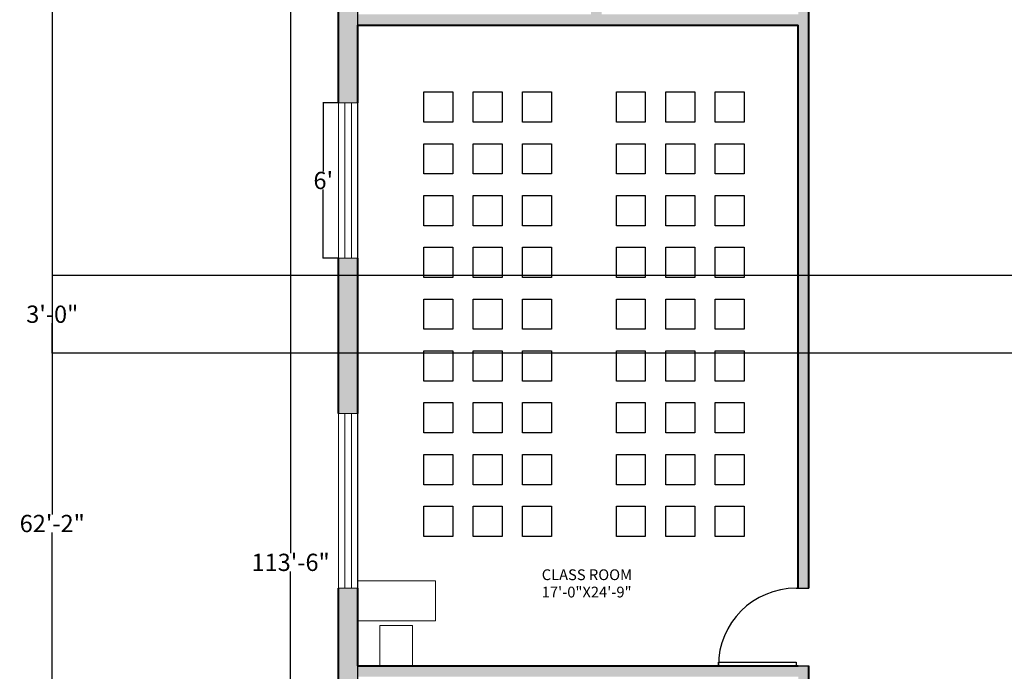
# Model space of a CAD drawing. Units: inches. Extents: x -405 to 940, y 226 to 2032.
# Tile 4 of 10: x -405 to 51, y 1156 to 1458. Entities that reach past the tile are written whole.
import ezdxf

# ---------------------------------------------------------------- set-up
doc = ezdxf.new("R2010")
doc.units = ezdxf.units.IN
doc.header["$MEASUREMENT"] = 0
doc.linetypes.add('ACAD_ISO02W100', pattern=[15, 12, -3])
for name, color, linetype, lineweight in [('A-ANNO-DIMS', 120, 'Continuous', 18), ('A-AREA-IDEN', 32, 'Continuous', 18), ('A-FURN-SEAT', 5, 'Continuous', 18), ('A-GLAZ-HIDN', 1, 'ACAD_ISO02W100', 18), ('A-WALL-PATT', 8, 'Continuous', 13), ('door', 6, 'Continuous', 25), ('tables', 2, 'Continuous', 18), ('wall', 3, 'Continuous', 40), ('window', 1, 'Continuous', 18)]:
    doc.layers.add(name, color=color, linetype=linetype, lineweight=lineweight)
doc.layers.add('beches', color=5, linetype='Continuous')
doc.styles.get("Standard").update_dxf_attribs({"font": 'arial.ttf'})
doc.dimstyles.get("Standard").update_dxf_attribs({"dimtxt": 8, "dimasz": 0.18, "dimexe": 0.18, "dimexo": 0.0625, "dimgap": 0.09, "dimtad": 0, "dimtih": 1, "dimtoh": 1, "dimdec": 0, "dimzin": 0, "dimdsep": 46, "dimlunit": 3, "dimtxsty": 'Standard', "dimblk": 'OBLIQUE', "dimcen": 0.09, "dimadec": 0, "dimazin": 0, "dimtfac": 1, "dimtdec": 0, "dimtofl": 0, "dimtmove": 0, "dimatfit": 3, "dimfxl": 1, "dimtolj": 1, "dimtzin": 0, "dimarcsym": 0})

# ---------------------------------------------------------------- blocks, each defined once
blk = doc.blocks.new('*U4')
for p, q in [((0, 0), (0, -6)), ((36, 0), (36, -6))]:
    blk.add_line(p, q)
blk.add_lwpolyline([(0, 0), (0, 36), (1.75, 36), (1.75, 0)], close=True)
blk.add_arc((0, 0), 36, 0, 90)
blk = doc.blocks.new('*U7')
at = {"layer": 'beches'}
blk.add_lwpolyline([(6.71, -7.02), (-6.71, -7.02), (-6.71, 7.02), (6.71, 7.02)], close=True, dxfattribs=at)
blk = doc.blocks.new('*U8')
at = {"layer": 'A-FURN-SEAT', "transparency": 16777216}
for p in [(-45.84, 192), (-45.84, 192, 12), (-45.84, 192, 24), (-45.84, 192, 36), (-45.84, 192, 48), (-45.84, 192, 60), (-45.84, 192, 72), (-45.84, 192, 84), (-45.84, 192, 96), (-45.84, 192, 108), (-45.84, 192, 120), (-45.84, 192, 132), (-22.92, 192), (-22.92, 192, 12), (-22.92, 192, 24), (-22.92, 192, 36), (-22.92, 192, 48), (-22.92, 192, 60), (-22.92, 192, 72), (-22.92, 192, 84), (-22.92, 192, 96), (-22.92, 192, 108), (-22.92, 192, 120), (-22.92, 192, 132), (0, 192), (0, 192, 12), (0, 192, 24), (0, 192, 36), (0, 192, 48), (0, 192, 60), (0, 192, 72), (0, 192, 84), (0, 192, 96), (0, 192, 108), (0, 192, 120), (0, 192, 132), (-45.84, 168), (-45.84, 168, 12), (-45.84, 168, 24), (-45.84, 168, 36), (-45.84, 168, 48), (-45.84, 168, 60), (-45.84, 168, 72), (-45.84, 168, 84), (-45.84, 168, 96), (-45.84, 168, 108), (-45.84, 168, 120), (-45.84, 168, 132), (-22.92, 168), (-22.92, 168, 12), (-22.92, 168, 24), (-22.92, 168, 36), (-22.92, 168, 48), (-22.92, 168, 60), (-22.92, 168, 72), (-22.92, 168, 84), (-22.92, 168, 96), (-22.92, 168, 108), (-22.92, 168, 120), (-22.92, 168, 132), (0, 168), (0, 168, 12), (0, 168, 24), (0, 168, 36), (0, 168, 48), (0, 168, 60), (0, 168, 72), (0, 168, 84), (0, 168, 96), (0, 168, 108), (0, 168, 120), (0, 168, 132), (-45.84, 144), (-45.84, 144, 12), (-45.84, 144, 24), (-45.84, 144, 36), (-45.84, 144, 48), (-45.84, 144, 60), (-45.84, 144, 72), (-45.84, 144, 84), (-45.84, 144, 96), (-45.84, 144, 108), (-45.84, 144, 120), (-45.84, 144, 132), (-22.92, 144), (-22.92, 144, 12), (-22.92, 144, 24), (-22.92, 144, 36), (-22.92, 144, 48), (-22.92, 144, 60), (-22.92, 144, 72), (-22.92, 144, 84), (-22.92, 144, 96), (-22.92, 144, 108), (-22.92, 144, 120), (-22.92, 144, 132), (0, 144), (0, 144, 12), (0, 144, 24), (0, 144, 36), (0, 144, 48), (0, 144, 60), (0, 144, 72), (0, 144, 84), (0, 144, 96), (0, 144, 108), (0, 144, 120), (0, 144, 132), (-45.84, 120), (-45.84, 120, 12), (-45.84, 120, 24), (-45.84, 120, 36), (-45.84, 120, 48), (-45.84, 120, 60), (-45.84, 120, 72), (-45.84, 120, 84), (-45.84, 120, 96), (-45.84, 120, 108), (-45.84, 120, 120), (-45.84, 120, 132), (-22.92, 120), (-22.92, 120, 12), (-22.92, 120, 24), (-22.92, 120, 36), (-22.92, 120, 48), (-22.92, 120, 60), (-22.92, 120, 72), (-22.92, 120, 84), (-22.92, 120, 96), (-22.92, 120, 108), (-22.92, 120, 120), (-22.92, 120, 132), (0, 120), (0, 120, 12), (0, 120, 24), (0, 120, 36), (0, 120, 48), (0, 120, 60), (0, 120, 72), (0, 120, 84), (0, 120, 96), (0, 120, 108), (0, 120, 120), (0, 120, 132), (-45.84, 96), (-45.84, 96, 12), (-45.84, 96, 24), (-45.84, 96, 36), (-45.84, 96, 48), (-45.84, 96, 60), (-45.84, 96, 72), (-45.84, 96, 84), (-45.84, 96, 96), (-45.84, 96, 108), (-45.84, 96, 120), (-45.84, 96, 132), (-22.92, 96), (-22.92, 96, 12), (-22.92, 96, 24), (-22.92, 96, 36), (-22.92, 96, 48), (-22.92, 96, 60), (-22.92, 96, 72), (-22.92, 96, 84), (-22.92, 96, 96), (-22.92, 96, 108), (-22.92, 96, 120), (-22.92, 96, 132), (0, 96), (0, 96, 12), (0, 96, 24), (0, 96, 36), (0, 96, 48), (0, 96, 60), (0, 96, 72), (0, 96, 84), (0, 96, 96), (0, 96, 108), (0, 96, 120), (0, 96, 132), (-45.84, 72), (-45.84, 72, 12), (-45.84, 72, 24), (-45.84, 72, 36), (-45.84, 72, 48), (-45.84, 72, 60), (-45.84, 72, 72), (-45.84, 72, 84), (-45.84, 72, 96), (-45.84, 72, 108), (-45.84, 72, 120), (-45.84, 72, 132), (-22.92, 72), (-22.92, 72, 12), (-22.92, 72, 24), (-22.92, 72, 36), (-22.92, 72, 48), (-22.92, 72, 60), (-22.92, 72, 72), (-22.92, 72, 84), (-22.92, 72, 96), (-22.92, 72, 108), (-22.92, 72, 120), (-22.92, 72, 132), (0, 72), (0, 72, 12), (0, 72, 24), (0, 72, 36), (0, 72, 48), (0, 72, 60), (0, 72, 72), (0, 72, 84), (0, 72, 96), (0, 72, 108), (0, 72, 120), (0, 72, 132), (-45.84, 48), (-45.84, 48, 12), (-45.84, 48, 24), (-45.84, 48, 36), (-45.84, 48, 48), (-45.84, 48, 60), (-45.84, 48, 72), (-45.84, 48, 84), (-45.84, 48, 96), (-45.84, 48, 108), (-45.84, 48, 120), (-45.84, 48, 132), (-22.92, 48), (-22.92, 48, 12), (-22.92, 48, 24), (-22.92, 48, 36), (-22.92, 48, 48), (-22.92, 48, 60), (-22.92, 48, 72), (-22.92, 48, 84), (-22.92, 48, 96), (-22.92, 48, 108), (-22.92, 48, 120), (-22.92, 48, 132), (0, 48), (0, 48, 12), (0, 48, 24), (0, 48, 36), (0, 48, 48), (0, 48, 60), (0, 48, 72), (0, 48, 84), (0, 48, 96), (0, 48, 108), (0, 48, 120), (0, 48, 132), (-45.84, 24), (-45.84, 24, 12), (-45.84, 24, 24), (-45.84, 24, 36), (-45.84, 24, 48), (-45.84, 24, 60), (-45.84, 24, 72), (-45.84, 24, 84), (-45.84, 24, 96), (-45.84, 24, 108), (-45.84, 24, 120), (-45.84, 24, 132), (-22.92, 24), (-22.92, 24, 12), (-22.92, 24, 24), (-22.92, 24, 36), (-22.92, 24, 48), (-22.92, 24, 60), (-22.92, 24, 72), (-22.92, 24, 84), (-22.92, 24, 96), (-22.92, 24, 108), (-22.92, 24, 120), (-22.92, 24, 132), (0, 24), (0, 24, 12), (0, 24, 24), (0, 24, 36), (0, 24, 48), (0, 24, 60), (0, 24, 72), (0, 24, 84), (0, 24, 96), (0, 24, 108), (0, 24, 120), (0, 24, 132), (-45.84, 0), (-45.84, 0, 12), (-45.84, 0, 24), (-45.84, 0, 36), (-45.84, 0, 48), (-45.84, 0, 60), (-45.84, 0, 72), (-45.84, 0, 84), (-45.84, 0, 96), (-45.84, 0, 108), (-45.84, 0, 120), (-45.84, 0, 132), (-22.92, 0), (-22.92, 0, 12), (-22.92, 0, 24), (-22.92, 0, 36), (-22.92, 0, 48), (-22.92, 0, 60), (-22.92, 0, 72), (-22.92, 0, 84), (-22.92, 0, 96), (-22.92, 0, 108), (-22.92, 0, 120), (-22.92, 0, 132), (0, 0), (0, 0, 12), (0, 0, 24), (0, 0, 36), (0, 0, 48), (0, 0, 60), (0, 0, 72), (0, 0, 84), (0, 0, 96), (0, 0, 108), (0, 0, 120), (0, 0, 132)]:
    blk.add_blockref('*U7', p, dxfattribs=at)
blk = doc.blocks.new('*U9')
at = {"layer": 'beches'}
blk.add_lwpolyline([(6.71, -7.02), (-6.71, -7.02), (-6.71, 7.02), (6.71, 7.02)], close=True, dxfattribs=at)
blk = doc.blocks.new('*U10')
at = {"layer": 'A-FURN-SEAT', "transparency": 16777216}
for p in [(-45.84, 192), (-45.84, 192, 12), (-45.84, 192, 24), (-45.84, 192, 36), (-45.84, 192, 48), (-45.84, 192, 60), (-45.84, 192, 72), (-45.84, 192, 84), (-45.84, 192, 96), (-45.84, 192, 108), (-45.84, 192, 120), (-45.84, 192, 132), (-22.92, 192), (-22.92, 192, 12), (-22.92, 192, 24), (-22.92, 192, 36), (-22.92, 192, 48), (-22.92, 192, 60), (-22.92, 192, 72), (-22.92, 192, 84), (-22.92, 192, 96), (-22.92, 192, 108), (-22.92, 192, 120), (-22.92, 192, 132), (0, 192), (0, 192, 12), (0, 192, 24), (0, 192, 36), (0, 192, 48), (0, 192, 60), (0, 192, 72), (0, 192, 84), (0, 192, 96), (0, 192, 108), (0, 192, 120), (0, 192, 132), (-45.84, 168), (-45.84, 168, 12), (-45.84, 168, 24), (-45.84, 168, 36), (-45.84, 168, 48), (-45.84, 168, 60), (-45.84, 168, 72), (-45.84, 168, 84), (-45.84, 168, 96), (-45.84, 168, 108), (-45.84, 168, 120), (-45.84, 168, 132), (-22.92, 168), (-22.92, 168, 12), (-22.92, 168, 24), (-22.92, 168, 36), (-22.92, 168, 48), (-22.92, 168, 60), (-22.92, 168, 72), (-22.92, 168, 84), (-22.92, 168, 96), (-22.92, 168, 108), (-22.92, 168, 120), (-22.92, 168, 132), (0, 168), (0, 168, 12), (0, 168, 24), (0, 168, 36), (0, 168, 48), (0, 168, 60), (0, 168, 72), (0, 168, 84), (0, 168, 96), (0, 168, 108), (0, 168, 120), (0, 168, 132), (-45.84, 144), (-45.84, 144, 12), (-45.84, 144, 24), (-45.84, 144, 36), (-45.84, 144, 48), (-45.84, 144, 60), (-45.84, 144, 72), (-45.84, 144, 84), (-45.84, 144, 96), (-45.84, 144, 108), (-45.84, 144, 120), (-45.84, 144, 132), (-22.92, 144), (-22.92, 144, 12), (-22.92, 144, 24), (-22.92, 144, 36), (-22.92, 144, 48), (-22.92, 144, 60), (-22.92, 144, 72), (-22.92, 144, 84), (-22.92, 144, 96), (-22.92, 144, 108), (-22.92, 144, 120), (-22.92, 144, 132), (0, 144), (0, 144, 12), (0, 144, 24), (0, 144, 36), (0, 144, 48), (0, 144, 60), (0, 144, 72), (0, 144, 84), (0, 144, 96), (0, 144, 108), (0, 144, 120), (0, 144, 132), (-45.84, 120), (-45.84, 120, 12), (-45.84, 120, 24), (-45.84, 120, 36), (-45.84, 120, 48), (-45.84, 120, 60), (-45.84, 120, 72), (-45.84, 120, 84), (-45.84, 120, 96), (-45.84, 120, 108), (-45.84, 120, 120), (-45.84, 120, 132), (-22.92, 120), (-22.92, 120, 12), (-22.92, 120, 24), (-22.92, 120, 36), (-22.92, 120, 48), (-22.92, 120, 60), (-22.92, 120, 72), (-22.92, 120, 84), (-22.92, 120, 96), (-22.92, 120, 108), (-22.92, 120, 120), (-22.92, 120, 132), (0, 120), (0, 120, 12), (0, 120, 24), (0, 120, 36), (0, 120, 48), (0, 120, 60), (0, 120, 72), (0, 120, 84), (0, 120, 96), (0, 120, 108), (0, 120, 120), (0, 120, 132), (-45.84, 96), (-45.84, 96, 12), (-45.84, 96, 24), (-45.84, 96, 36), (-45.84, 96, 48), (-45.84, 96, 60), (-45.84, 96, 72), (-45.84, 96, 84), (-45.84, 96, 96), (-45.84, 96, 108), (-45.84, 96, 120), (-45.84, 96, 132), (-22.92, 96), (-22.92, 96, 12), (-22.92, 96, 24), (-22.92, 96, 36), (-22.92, 96, 48), (-22.92, 96, 60), (-22.92, 96, 72), (-22.92, 96, 84), (-22.92, 96, 96), (-22.92, 96, 108), (-22.92, 96, 120), (-22.92, 96, 132), (0, 96), (0, 96, 12), (0, 96, 24), (0, 96, 36), (0, 96, 48), (0, 96, 60), (0, 96, 72), (0, 96, 84), (0, 96, 96), (0, 96, 108), (0, 96, 120), (0, 96, 132), (-45.84, 72), (-45.84, 72, 12), (-45.84, 72, 24), (-45.84, 72, 36), (-45.84, 72, 48), (-45.84, 72, 60), (-45.84, 72, 72), (-45.84, 72, 84), (-45.84, 72, 96), (-45.84, 72, 108), (-45.84, 72, 120), (-45.84, 72, 132), (-22.92, 72), (-22.92, 72, 12), (-22.92, 72, 24), (-22.92, 72, 36), (-22.92, 72, 48), (-22.92, 72, 60), (-22.92, 72, 72), (-22.92, 72, 84), (-22.92, 72, 96), (-22.92, 72, 108), (-22.92, 72, 120), (-22.92, 72, 132), (0, 72), (0, 72, 12), (0, 72, 24), (0, 72, 36), (0, 72, 48), (0, 72, 60), (0, 72, 72), (0, 72, 84), (0, 72, 96), (0, 72, 108), (0, 72, 120), (0, 72, 132), (-45.84, 48), (-45.84, 48, 12), (-45.84, 48, 24), (-45.84, 48, 36), (-45.84, 48, 48), (-45.84, 48, 60), (-45.84, 48, 72), (-45.84, 48, 84), (-45.84, 48, 96), (-45.84, 48, 108), (-45.84, 48, 120), (-45.84, 48, 132), (-22.92, 48), (-22.92, 48, 12), (-22.92, 48, 24), (-22.92, 48, 36), (-22.92, 48, 48), (-22.92, 48, 60), (-22.92, 48, 72), (-22.92, 48, 84), (-22.92, 48, 96), (-22.92, 48, 108), (-22.92, 48, 120), (-22.92, 48, 132), (0, 48), (0, 48, 12), (0, 48, 24), (0, 48, 36), (0, 48, 48), (0, 48, 60), (0, 48, 72), (0, 48, 84), (0, 48, 96), (0, 48, 108), (0, 48, 120), (0, 48, 132), (-45.84, 24), (-45.84, 24, 12), (-45.84, 24, 24), (-45.84, 24, 36), (-45.84, 24, 48), (-45.84, 24, 60), (-45.84, 24, 72), (-45.84, 24, 84), (-45.84, 24, 96), (-45.84, 24, 108), (-45.84, 24, 120), (-45.84, 24, 132), (-22.92, 24), (-22.92, 24, 12), (-22.92, 24, 24), (-22.92, 24, 36), (-22.92, 24, 48), (-22.92, 24, 60), (-22.92, 24, 72), (-22.92, 24, 84), (-22.92, 24, 96), (-22.92, 24, 108), (-22.92, 24, 120), (-22.92, 24, 132), (0, 24), (0, 24, 12), (0, 24, 24), (0, 24, 36), (0, 24, 48), (0, 24, 60), (0, 24, 72), (0, 24, 84), (0, 24, 96), (0, 24, 108), (0, 24, 120), (0, 24, 132), (-45.84, 0), (-45.84, 0, 12), (-45.84, 0, 24), (-45.84, 0, 36), (-45.84, 0, 48), (-45.84, 0, 60), (-45.84, 0, 72), (-45.84, 0, 84), (-45.84, 0, 96), (-45.84, 0, 108), (-45.84, 0, 120), (-45.84, 0, 132), (-22.92, 0), (-22.92, 0, 12), (-22.92, 0, 24), (-22.92, 0, 36), (-22.92, 0, 48), (-22.92, 0, 60), (-22.92, 0, 72), (-22.92, 0, 84), (-22.92, 0, 96), (-22.92, 0, 108), (-22.92, 0, 120), (-22.92, 0, 132), (0, 0), (0, 0, 12), (0, 0, 24), (0, 0, 36), (0, 0, 48), (0, 0, 60), (0, 0, 72), (0, 0, 84), (0, 0, 96), (0, 0, 108), (0, 0, 120), (0, 0, 132)]:
    blk.add_blockref('*U9', p, dxfattribs=at)
blk = doc.blocks.new('_Oblique')
at = {"color": 0, "linetype": 'ByBlock', "lineweight": -2}
blk.add_line((-0.5, -0.5), (0.5, 0.5), dxfattribs=at)
blk = doc.blocks.new('*D44')
at = {"layer": 'A-ANNO-DIMS', "color": 0, "lineweight": -2, "transparency": 16777216}
for p, q in [((-257.29, 1887.81), (-279.61, 1887.81)), ((-279.43, 1887.81), (-279.43, 1210.99)), ((-279.43, 525.81), (-279.43, 1202.63)), ((-257.29, 525.81), (-279.61, 525.81))]:
    blk.add_line(p, q, dxfattribs=at)
at = {"layer": 'Defpoints', "color": 0, "transparency": 16777216}
for p in [(-257.23, 1887.81), (-279.43, 525.81), (-257.23, 525.81)]:
    blk.add_point(p, dxfattribs=at)
at = {"layer": 'A-ANNO-DIMS', "color": 0, "lineweight": -2, "transparency": 16777216, "xscale": 0.18, "yscale": 0.18, "zscale": 0.18}
for p, rotation in [((-279.43, 1887.81), 90), ((-279.43, 525.81), 270)]:
    blk.add_blockref('_Oblique', p, dxfattribs=dict(at, rotation=rotation))
at = {"layer": 'A-ANNO-DIMS', "color": 0, "transparency": 16777216, "insert": (-279.43, 1206.81), "char_height": 8, "attachment_point": 5}
blk.add_mtext('\\A1;113\'-6"', dxfattribs=at)
blk = doc.blocks.new('*D55')
at = {"layer": 'A-ANNO-DIMS', "color": 0, "lineweight": -2, "transparency": 16777216}
for p, q in [((-257.29, 1419.81), (-264.48, 1419.81)), ((-264.3, 1419.81), (-264.3, 1387.98)), ((-264.3, 1347.81), (-264.3, 1379.64)), ((-257.29, 1347.81), (-264.48, 1347.81))]:
    blk.add_line(p, q, dxfattribs=at)
at = {"layer": 'Defpoints', "color": 0, "transparency": 16777216}
for p in [(-264.3, 1419.81), (-257.23, 1419.81), (-257.23, 1347.81)]:
    blk.add_point(p, dxfattribs=at)
at = {"layer": 'A-ANNO-DIMS', "color": 0, "lineweight": -2, "transparency": 16777216, "xscale": 0.18, "yscale": 0.18, "zscale": 0.18}
for p, rotation in [((-264.3, 1419.81), 90), ((-264.3, 1347.81), 270)]:
    blk.add_blockref('_Oblique', p, dxfattribs=dict(at, rotation=rotation))
at = {"layer": 'A-ANNO-DIMS', "color": 0, "transparency": 16777216, "insert": (-264.3, 1383.81), "char_height": 8, "attachment_point": 5}
blk.add_mtext("\\A1;6'", dxfattribs=at)
blk = doc.blocks.new('WIN-PANE-72IN')
for p, q in [((0, 3), (72, 3)), ((0, 0), (72, 0))]:
    blk.add_line(p, q)
blk = doc.blocks.new('*D107')
at = {"layer": 'A-ANNO-DIMS', "color": 0, "lineweight": -2, "transparency": 16777216}
for p, q in [((501.71, 1597.81), (-390.06, 1597.81)), ((-389.88, 1597.81), (-389.88, 1228.98)), ((-389.88, 851.81), (-389.88, 1220.64)), ((501.71, 851.81), (-390.06, 851.81))]:
    blk.add_line(p, q, dxfattribs=at)
at = {"layer": 'Defpoints', "color": 0, "transparency": 16777216}
for p in [(-389.88, 1597.81), (501.77, 1597.81), (501.77, 851.81)]:
    blk.add_point(p, dxfattribs=at)
at = {"layer": 'A-ANNO-DIMS', "color": 0, "lineweight": -2, "transparency": 16777216, "xscale": 0.18, "yscale": 0.18, "zscale": 0.18}
for p, rotation in [((-389.88, 1597.81), 90), ((-389.88, 851.81), 270)]:
    blk.add_blockref('_Oblique', p, dxfattribs=dict(at, rotation=rotation))
at = {"layer": 'A-ANNO-DIMS', "color": 0, "transparency": 16777216, "insert": (-389.88, 1224.81), "char_height": 8, "attachment_point": 5}
blk.add_mtext('\\A1;62\'-2"', dxfattribs=at)
blk = doc.blocks.new('*D109')
at = {"layer": 'A-ANNO-DIMS', "color": 0, "lineweight": -2, "transparency": 16777216}
for p, q in [((-248.23, 750.87), (-248.23, 2020.64)), ((-248.23, 2020.46), (-49.06, 2020.46)), ((177.77, 2020.46), (-21.4, 2020.46)), ((177.77, 750.87), (177.77, 2020.64))]:
    blk.add_line(p, q, dxfattribs=at)
at = {"layer": 'Defpoints', "color": 0, "transparency": 16777216}
for p in [(177.77, 2020.46), (-248.23, 750.81), (177.77, 750.81)]:
    blk.add_point(p, dxfattribs=at)
at = {"layer": 'A-ANNO-DIMS', "color": 0, "lineweight": -2, "transparency": 16777216, "xscale": 0.18, "yscale": 0.18, "zscale": 0.18, "rotation": 180}
blk.add_blockref('_Oblique', (-248.23, 2020.46), dxfattribs=at)
at = {"layer": 'A-ANNO-DIMS', "color": 0, "lineweight": -2, "transparency": 16777216, "xscale": 0.18, "yscale": 0.18, "zscale": 0.18}
blk.add_blockref('_Oblique', (177.77, 2020.46), dxfattribs=at)
at = {"layer": 'A-ANNO-DIMS', "color": 0, "transparency": 16777216, "insert": (-35.23, 2020.46), "char_height": 8, "attachment_point": 5}
blk.add_mtext('\\A1;35\'-6"', dxfattribs=at)
blk = doc.blocks.new('*D114')
at = {"layer": 'A-ANNO-DIMS', "color": 0, "lineweight": -2, "transparency": 16777216}
for p, q in [((602.71, 1339.81), (-390.06, 1339.81)), ((-389.88, 1339.81), (-389.88, 1325.99)), ((-389.88, 1303.81), (-389.88, 1317.63)), ((602.71, 1303.81), (-390.06, 1303.81))]:
    blk.add_line(p, q, dxfattribs=at)
at = {"layer": 'Defpoints', "color": 0, "transparency": 16777216}
for p in [(602.77, 1339.81), (-389.88, 1303.81), (602.77, 1303.81)]:
    blk.add_point(p, dxfattribs=at)
at = {"layer": 'A-ANNO-DIMS', "color": 0, "lineweight": -2, "transparency": 16777216, "xscale": 0.18, "yscale": 0.18, "zscale": 0.18}
for p, rotation in [((-389.88, 1339.81), 90), ((-389.88, 1303.81), 270)]:
    blk.add_blockref('_Oblique', p, dxfattribs=dict(at, rotation=rotation))
at = {"layer": 'A-ANNO-DIMS', "color": 0, "transparency": 16777216, "insert": (-389.88, 1321.81), "char_height": 8, "attachment_point": 5}
blk.add_mtext('\\A1;3\'-0"', dxfattribs=at)

msp = doc.modelspace()

# ---------------------------------------------------------------- hatches: boundary and pattern name
at = {"layer": 'A-WALL-PATT'}
h = msp.add_hatch(dxfattribs=at)
h.set_pattern_fill('AR-HBONE', color=256)
h.set_pattern_definition([(45, (599.8442, 904.9158), (0, 5.656854), [12, -4]), (135, (602.6726, 907.744), (4e-16, 5.656854), [12, -4])])
h.paths.add_polyline_path([(-248.23, 1045.81), (-257.23, 1045.81), (-257.23, 964.81), (-248.23, 964.81)], flags=17)
h.paths.add_polyline_path([(-248.23, 851.81), (-39.23, 851.81), (-39.23, 856.81), (-44.23, 856.81), (-248.23, 856.81), (-248.23, 892.81), (-257.23, 892.81), (-257.23, 839.81), (-248.23, 839.81)])
h.paths.add_polyline_path([(-248.23, 750.81), (124.74, 750.81), (124.74, 751.73), (124.74, 755.81), (-248.23, 755.81), (-248.23, 767.81), (-257.23, 767.81), (-257.23, 726.81), (-248.23, 726.81)])
h.paths.add_polyline_path([(-248.23, 654.81), (-257.23, 654.81), (-257.23, 630.81), (-248.23, 630.81)])
h.paths.add_polyline_path([(-180.23, 534.81), (-248.23, 534.81), (-248.23, 558.81), (-257.23, 558.81), (-257.23, 525.81), (-180.23, 525.81)])
h.paths.add_polyline_path([(-69.23, 534.81), (-108.23, 534.81), (-108.23, 525.81), (-69.23, 525.81)])
h.paths.add_polyline_path([(35.77, 534.81), (2.77, 534.81), (2.77, 525.81), (35.77, 525.81)])
h.paths.add_polyline_path([(182.77, 755.81), (160.74, 755.81), (160.74, 750.81), (177.77, 750.81), (177.77, 534.81), (107.77, 534.81), (107.77, 525.81), (182.77, 525.81)])
h.paths.add_polyline_path([(-39.23, 1609.81), (-44.23, 1609.81), (-44.23, 1604.81), (-44.23, 1460.81), (-135.23, 1460.81), (-135.23, 1465.73), (-140.23, 1465.73), (-140.23, 1460.81), (-248.23, 1460.81), (-248.23, 1471.31), (-257.23, 1471.31), (-257.23, 1419.81), (-248.23, 1419.81), (-248.23, 1455.81), (-44.23, 1455.81), (-44.23, 1194.81), (-39.23, 1194.81)])
h.paths.add_polyline_path([(-248.23, 1520.81), (-257.23, 1520.81), (-257.23, 1495.31), (-248.23, 1495.31), (-248.23, 1505.81), (-140.23, 1505.81), (-140.23, 1495.73), (-135.23, 1495.73), (-135.23, 1516.79), (-140.23, 1516.79), (-140.23, 1510.81), (-248.23, 1510.81)], flags=17)
h.paths.add_polyline_path([(-248.23, 1570.31), (-257.23, 1570.31), (-257.23, 1544.81), (-248.23, 1544.81), (-248.23, 1554.81), (-140.23, 1554.81), (-140.23, 1546.79), (-135.23, 1546.79), (-135.23, 1565.08), (-140.23, 1565.08), (-140.23, 1559.81), (-248.23, 1559.81)], flags=17)
h.paths.add_polyline_path([(-248.23, 1615.81), (-257.23, 1615.81), (-257.23, 1594.31), (-248.23, 1594.31), (-248.23, 1604.81), (-140.23, 1604.81), (-140.23, 1595.08), (-135.23, 1595.08), (-135.23, 1604.81), (-80.23, 1604.81), (-80.23, 1609.81), (-248.23, 1609.81)])
h.paths.add_polyline_path([(-248.23, 1783.81), (-235.46, 1783.81), (-235.46, 1788.81), (-248.23, 1788.81), (-248.23, 1878.81), (-237.73, 1878.81), (-237.73, 1887.81), (-257.23, 1887.81), (-257.23, 1687.81), (-248.23, 1687.81), (-248.23, 1693.81), (-136.23, 1693.81), (-136.23, 1698.81), (-248.23, 1698.81)])
h.paths.add_polyline_path([(-188.23, 1887.81), (-213.73, 1887.81), (-213.73, 1878.81), (-203.23, 1878.81), (-203.23, 1788.81), (-205.46, 1788.81), (-205.46, 1783.81), (-186.39, 1783.81), (-186.39, 1788.81), (-198.23, 1788.81), (-198.23, 1878.81), (-188.23, 1878.81)])
h.paths.add_polyline_path([(-139.23, 1887.81), (-164.23, 1887.81), (-164.23, 1878.81), (-154.23, 1878.81), (-154.23, 1788.81), (-156.39, 1788.81), (-156.39, 1783.81), (-138.25, 1783.81), (-138.25, 1788.81), (-149.23, 1788.81), (-149.23, 1878.81), (-139.23, 1878.81)])
h.paths.add_polyline_path([(-89.23, 1887.81), (-115.23, 1887.81), (-115.23, 1878.81), (-105.23, 1878.81), (-105.23, 1788.81), (-108.25, 1788.81), (-108.25, 1783.81), (-86.45, 1783.81), (-86.45, 1788.81), (-100.23, 1788.81), (-100.23, 1878.81), (-89.23, 1878.81)])
h.paths.add_polyline_path([(-36.23, 1887.81), (-65.23, 1887.81), (-65.23, 1878.81), (-54.23, 1878.81), (-54.23, 1788.81), (-56.45, 1788.81), (-56.45, 1783.81), (-54.23, 1783.81), (-54.23, 1698.81), (-100.23, 1698.81), (-100.23, 1693.81), (-49.23, 1693.81), (-49.23, 1698.81), (-49.23, 1878.81), (-36.23, 1878.81)])
h.paths.add_polyline_path([(89.77, 1887.81), (35.77, 1887.81), (35.77, 1878.81), (48.77, 1878.81), (48.77, 1698.81), (-13.23, 1698.81), (-13.23, 1693.81), (53.77, 1693.81), (53.77, 1698.81), (53.77, 1878.81), (89.77, 1878.81)])
h.paths.add_polyline_path([(255.27, 1887.81), (161.77, 1887.81), (161.77, 1878.81), (197.77, 1878.81), (197.77, 1698.81), (89.77, 1698.81), (89.77, 1693.81), (202.77, 1693.81), (202.77, 1698.81), (202.77, 1878.81), (255.27, 1878.81)])
h.paths.add_polyline_path([(375.27, 1887.81), (327.27, 1887.81), (327.27, 1878.81), (375.27, 1878.81)], flags=17)
h.paths.add_polyline_path([(815.77, 1887.81), (447.27, 1887.81), (447.27, 1878.81), (499.77, 1878.81), (499.77, 1698.81), (238.77, 1698.81), (238.77, 1693.81), (504.77, 1693.81), (504.77, 1878.81), (633.77, 1878.81), (633.77, 1646.81), (597.77, 1646.81), (597.77, 1641.81), (602.77, 1641.81), (638.77, 1641.81), (638.77, 1878.81), (806.77, 1878.81), (806.77, 1838.31), (815.77, 1838.31)])
h.paths.add_polyline_path([(815.77, 1766.31), (806.77, 1766.31), (806.77, 1718.31), (815.77, 1718.31)], flags=17)
h.paths.add_polyline_path([(815.77, 1356.31), (806.77, 1356.31), (806.77, 1303.81), (602.77, 1303.81), (597.77, 1303.81), (597.77, 1037.81), (602.77, 1037.81), (602.77, 1298.81), (806.77, 1298.81), (806.77, 1246.31), (815.77, 1246.31)])
h.paths.add_polyline_path([(815.77, 1174.31), (806.77, 1174.31), (806.77, 1126.31), (815.77, 1126.31)], flags=17)
h.paths.add_polyline_path([(815.77, 1054.31), (806.77, 1054.31), (806.77, 1001.81), (796.08, 1001.81), (796.08, 1001.75), (780.86, 1001.75), (602.77, 1001.81), (597.77, 1001.81), (597.77, 892.81), (602.77, 892.81), (602.77, 996.81), (806.77, 996.81), (806.77, 962.81), (815.77, 962.81)])
h.paths.add_polyline_path([(403.77, 534.81), (379.77, 534.81), (379.77, 525.81), (403.77, 525.81)])
h.paths.add_polyline_path([(-39.23, 1158.81), (-44.23, 1158.81), (-248.23, 1158.81), (-248.23, 1194.81), (-257.23, 1194.81), (-257.23, 1117.81), (-248.23, 1117.81), (-248.23, 1153.81), (-44.23, 1153.81), (-44.23, 892.81), (-39.23, 892.81)])
h.paths.add_polyline_path([(-248.23, 1347.81), (-257.23, 1347.81), (-257.23, 1275.81), (-248.23, 1275.81)], flags=17)
h.paths.add_polyline_path([(815.77, 1476.31), (806.77, 1476.31), (806.77, 1428.31), (815.77, 1428.31)], flags=17)
h.paths.add_polyline_path([(815.77, 1646.31), (806.77, 1646.31), (806.77, 1638.65), (806.77, 1605.81), (597.77, 1605.81), (597.77, 1339.81), (602.77, 1339.81), (602.77, 1600.81), (806.77, 1600.81), (806.77, 1548.31), (815.77, 1548.31)])

# ---------------------------------------------------------------- linework, layer by layer
at = {"layer": 'A-FURN-SEAT'}
msp.add_lwpolyline([(-238.14, 1158.81), (-238.14, 1177.54), (-222.92, 1177.54), (-222.92, 1158.81)], close=True, dxfattribs=at)
at = {"layer": 'A-GLAZ-HIDN'}
for p, q in [((-248.23, 1419.81), (-257.23, 1419.81)), ((-248.23, 1347.81), (-257.23, 1347.81)), ((-248.23, 1275.81), (-257.23, 1275.81)), ((-248.23, 1194.81), (-257.23, 1194.81))]:
    msp.add_line(p, q, dxfattribs=at)
at = {"layer": 'door'}
for p, q in [((-44.23, 1194.81), (-39.23, 1194.81)), ((-44.23, 1158.81), (-39.23, 1158.81))]:
    msp.add_line(p, q, dxfattribs=at)
at = {"layer": 'tables'}
for p, q in [((-248.23, 1179.65), (-248.23, 1198.26)), ((-248.23, 1198.26), (-212.23, 1198.26)), ((-212.23, 1198.26), (-212.23, 1179.65)), ((-212.23, 1179.65), (-248.23, 1179.65))]:
    msp.add_line(p, q, dxfattribs=at)
at = {"layer": 'wall'}
for p, q in [((-39.23, 1194.81), (-39.23, 1609.81)), ((-257.23, 1419.81), (-257.23, 1471.31)), ((-248.23, 1455.81), (-44.23, 1455.81)), ((-248.23, 1419.81), (-248.23, 1455.81)), ((-44.23, 1194.81), (-44.23, 1455.81)), ((-257.23, 1275.81), (-257.23, 1347.81)), ((-248.23, 1275.81), (-248.23, 1347.81)), ((-257.23, 1117.81), (-257.23, 1194.81)), ((-248.23, 1158.81), (-248.23, 1194.81)), ((-248.23, 1158.81), (-44.23, 1158.81)), ((-39.23, 892.81), (-39.23, 1158.81))]:
    msp.add_line(p, q, dxfattribs=at)
at = {"layer": 'window'}
for p, q in [((-257.23, 1347.81), (-257.23, 1419.81)), ((-248.23, 1347.81), (-248.23, 1419.81)), ((-257.23, 1194.81), (-257.23, 1275.81)), ((-254.23, 1194.81), (-254.23, 1275.81)), ((-251.23, 1194.81), (-251.23, 1275.81)), ((-248.23, 1194.81), (-248.23, 1275.81))]:
    msp.add_line(p, q, dxfattribs=at)

# ---------------------------------------------------------------- block references
at = {"layer": 'A-FURN-SEAT'}
for name, p in [('*U10', (-165.21, 1225.83)), ('*U8', (-75.94, 1225.83))]:
    msp.add_blockref(name, p, dxfattribs=at)
at = {"layer": 'door', "rotation": 90}
msp.add_blockref('*U4', (-45.23, 1158.81), dxfattribs=at)
at = {"layer": 'window', "rotation": 90.0000000000001}
msp.add_blockref('WIN-PANE-72IN', (-251.23, 1347.81), dxfattribs=at)

# ---------------------------------------------------------------- texts
at = {"layer": 'A-AREA-IDEN'}
for s, p in [('CLASS ROOM ', (-163.07, 1198.57)), ('17\'-0"X24\'-9"', (-163.07, 1190.54))]:
    msp.add_text(s, height=5, dxfattribs=at).set_placement(p)

# ---------------------------------------------------------------- dimensions: what is measured, and where the dimension line sits
at = {"layer": 'A-ANNO-DIMS'}
dim = msp.add_linear_dim(base=(177.77, 2020.46), p1=(-248.23, 750.81), p2=(177.77, 750.81), dimstyle='Standard', override={"dimdec": 1, "dimlfac": 1, "dimrnd": 0, "dimzin": 1, "dimdsep": 46, "dimlunit": 4, "dimfrac": 2}, dxfattribs=at)
dim.commit()
dim.dimension.update_dxf_attribs({"geometry": '*D109', "text_midpoint": (-35.23, 2020.46)})
for base, p1, p2, override, picture, middle in [((-279.43, 525.81), (-257.23, 1887.81), (-257.23, 525.81), {"dimclrd": 0, "dimclre": 0, "dimclrt": 0}, '*D44', (-279.43, 1206.81)), ((-389.88, 1597.81), (501.77, 851.81), (501.77, 1597.81), {"dimdec": 1, "dimlfac": 1, "dimrnd": 0, "dimzin": 1, "dimdsep": 46, "dimlunit": 4, "dimfrac": 2}, '*D107', (-389.88, 1224.81)), ((-264.3, 1419.81), (-257.23, 1347.81), (-257.23, 1419.81), {"dimclrd": 0, "dimclre": 0, "dimclrt": 0}, '*D55', (-264.3, 1383.81)), ((-389.88, 1303.81), (602.77, 1339.81), (602.77, 1303.81), {"dimdec": 1, "dimlfac": 1, "dimrnd": 0, "dimzin": 1, "dimdsep": 46, "dimlunit": 4, "dimfrac": 2}, '*D114', (-389.88, 1321.81))]:
    dim = msp.add_linear_dim(base=base, p1=p1, p2=p2, angle=90, dimstyle='Standard', override=override, dxfattribs=at)
    dim.commit()
    dim.dimension.update_dxf_attribs({"geometry": picture, "text_midpoint": middle})

doc.saveas('drawing.dxf')
